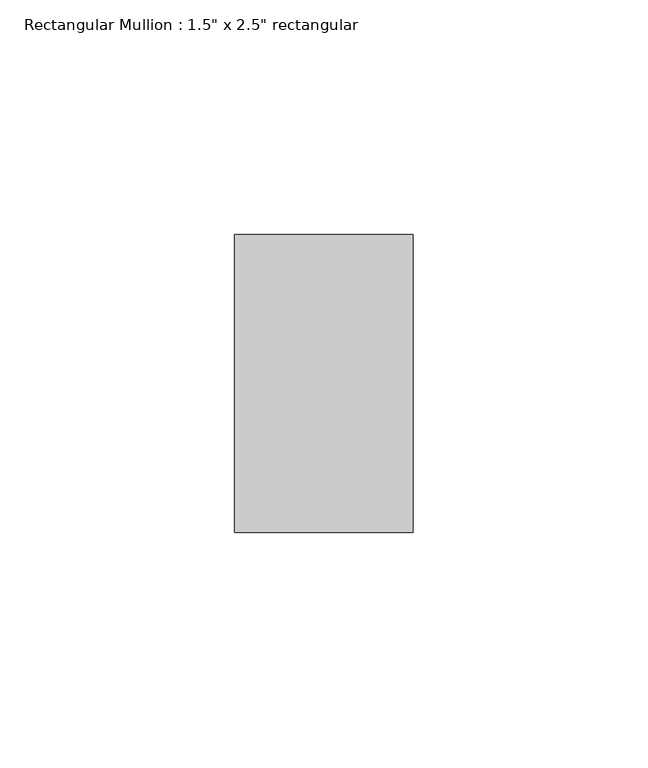
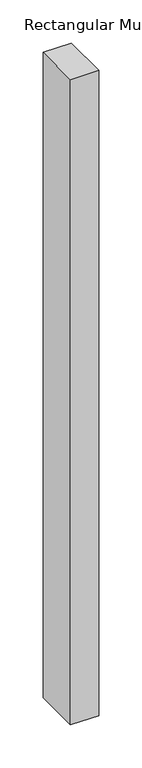
"""IFC4 building model written with IfcOpenShell, lengths in millimetres: member geometry."""

from ifc_helpers import new_model, si_unit, frame, origin, place, context, project, spatial, polyline, outline, extrude, source, transform, mapped, element, save


def member_c5b617ba(model_context):
    return source(origin(), model_context, "Body", "SweptSolid", [
        extrude(outline(polyline([(0.0, 31.75), (0.0, -31.75), (-38.1, -31.75), (-38.1, 31.75), (0.0, 31.75)])), frame((0.0, 0.0, -914.4), z_axis=(0.0, 0.0, 1.0), x_axis=(1.0, 0.0, 0.0)), (0.0, 0.0, 1.0), 914.4),
    ])


if __name__ == "__main__":
    model = new_model("IFC4")
    model_context = context("Model", 3, world=origin())
    ifc_project = project(units=[si_unit("LENGTHUNIT", "METRE", prefix="MILLI")], contexts=[model_context])
    site = spatial("IfcSite", under=ifc_project)
    building = spatial("IfcBuilding", under=site)
    placement = place(None, origin())
    member_shape = member_c5b617ba(model_context)
    element("IfcMember", 1, ObjectType="Rectangular Mullion : 1.5\" x 2.5\" rectangular", at=placement, inside=building, context=model_context, shape_type="MappedRepresentation", body=[
        mapped(member_shape, transform((0.0, 0.0, 0.0), x_axis=(1.0, 0.0, 0.0), y_axis=(0.0, 1.0, 0.0), z_axis=(0.0, 0.0, 1.0))),
    ])
    save(model, "model.ifc")

# Revit data of these elements
# Type "Rectangular Mullion : 1.5\" x 2.5\" rectangular"
#   built-in parameter 1007304 = 0.208333 (stored number, unit not read)
#   built-in parameter 1007301 = 0.0625 (stored number, unit not read)
#   built-in parameter 1007300 = 0.0625 (stored number, unit not read)
# Element 1 (IfcMember, "Rectangular Mullion : 1.5\" x 2.5\" rectangular")
#   Materials on its faces: "Aluminum"
# Materials
#   "Aluminum": class "Metal", colour RGB 247 247 247, transparency 0, Description = "Aluminum 6061", Cost = 0
